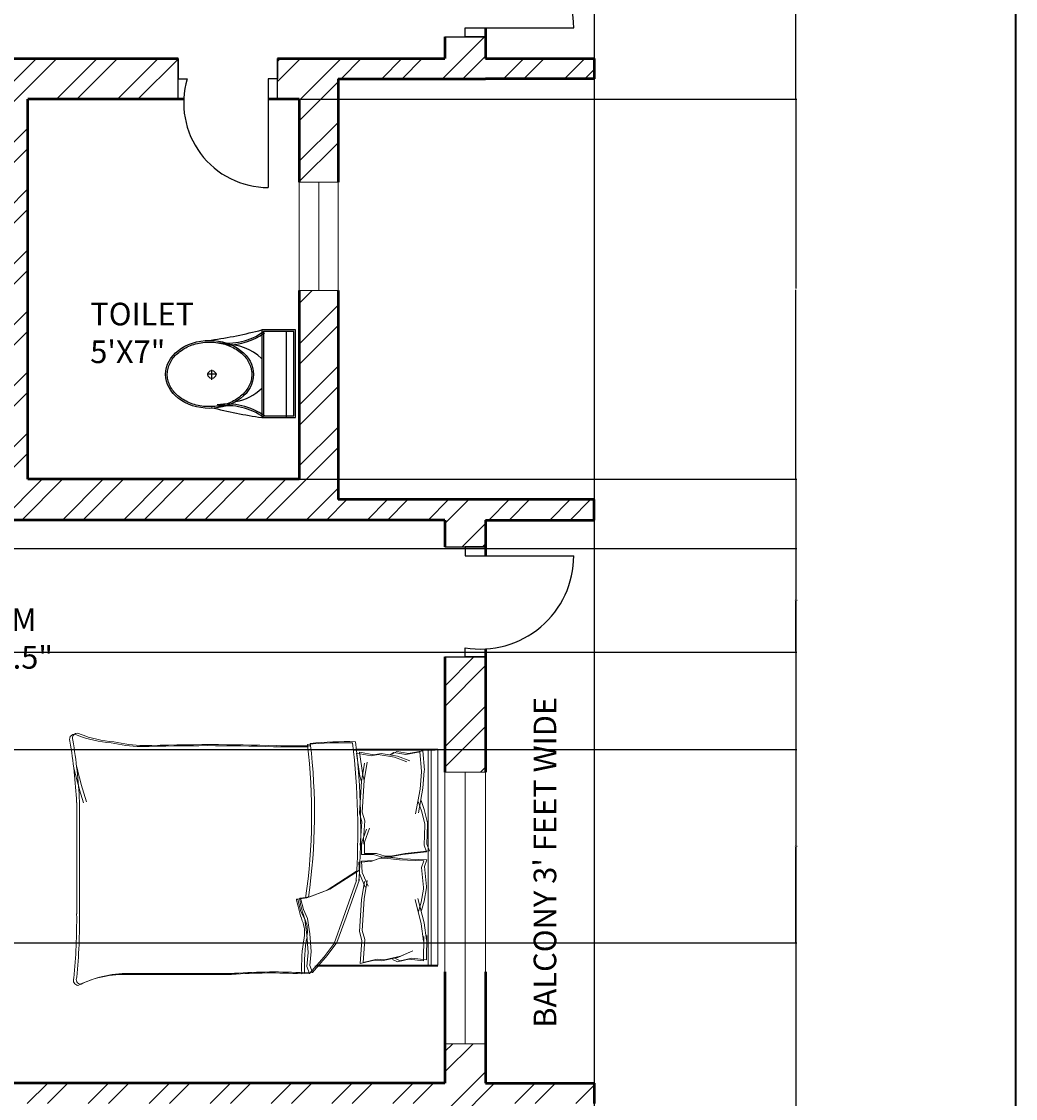
# Model space of a CAD drawing. Units: inches. Extents: x 1980 to 2738, y 1471 to 2568.
# Tile 15 of 22: x 2519 to 2738, y 1874 to 2112. Entities that reach past the tile are written whole.
import ezdxf

# ---------------------------------------------------------------- set-up
doc = ezdxf.new("R2010")
doc.units = ezdxf.units.IN
for name, color, linetype, lineweight in [('A-ANNO-DIMS', 2, 'Continuous', 18), ('A-ANNO-TTLB', 7, 'Continuous', 35), ('A-AREA-IDEN', 7, 'Continuous', 18), ('A-DOOR', 31, 'Continuous', 25), ('A-FLOR-BALC', 7, 'Continuous', 25), ('A-FLOR-FIXT', 8, 'Continuous', 25), ('A-FURN', 8, 'Continuous', 18), ('A-GLAZ', 141, 'Continuous', 18), ('A-WALL', 7, 'Continuous', 50)]:
    doc.layers.add(name, color=color, linetype=linetype, lineweight=lineweight)
doc.layers.add('A-WALL-PATT', color=9, linetype='Continuous', lineweight=13, true_color=0xd19cc7)
doc.styles.get("Standard").update_dxf_attribs({"font": 'arial.ttf'})
doc.dimstyles.get("Standard").update_dxf_attribs({"dimtxt": 0.18, "dimasz": 0.18, "dimexe": 0.18, "dimexo": 0.0625, "dimgap": 0.09, "dimtad": 0, "dimtih": 1, "dimtoh": 1, "dimdec": 4, "dimzin": 0, "dimdsep": 46, "dimtxsty": 'Standard', "dimcen": 0.09, "dimadec": 0, "dimazin": 0, "dimtfac": 1, "dimtdec": 4, "dimtofl": 0, "dimtmove": 0, "dimatfit": 3, "dimfxl": 1, "dimtolj": 1, "dimtzin": 0, "dimarcsym": 0})

# ---------------------------------------------------------------- blocks, each defined once
blk = doc.blocks.new('A$C31115884')
for p, q in [((257.5, 466.4), (257.5, 523.2)), ((283.1, 497.7), (223.4, 497.7)), ((0, 200), (0, 0)), ((520, 200), (0, 200)), ((520, 0), (520, 200)), ((10, 190), (10, 10)), ((510, 190), (10, 190)), ((510, 10), (510, 190)), ((510, 54.5), (0, 54.5)), ((10, 10), (510, 10)), ((0, 0), (520, 0))]:
    blk.add_line(p, q)
blk.add_circle((255.6, 496.4), 23.6)
for centre, radius, start, end in [((2777.7, -204.6), 2807, 165.4549, 171.71327), ((-294.5, 403.3), 364.7, 324.20913, 9.34987), ((-294.5, 403.3), 374.7, 324.20913, 9.34987), ((805.8, 403.3), 364.7, 170.65013, 215.79087), ((3237, 905), 2807, 188.28673, 194.5451), ((139.5, 406.2), 293.5, 315.84364, 2.65635), ((805.8, 403.3), 374.7, 179.20365, 215.79087), ((383.6, 406.2), 293.5, 190.27735, 224.15636)]:
    blk.add_arc(centre, radius, start, end)
blk.add_ellipse((256.2, 509.9), major_axis=(0, -260.7), ratio=0.772727)
blk.add_open_spline([(256.2, 259.2), (263.1, 259.2), (270, 259.7), (287.8, 262.3), (298.7, 265.1), (319.9, 273.1), (330.2, 278.4), (350.1, 291.1), (359.7, 298.7), (377.7, 315.9), (386.2, 325.5), (401.7, 346.6), (408.8, 358.1), (421.3, 382.5), (426.8, 395.5), (435.9, 422.4), (439.5, 436.4), (444.8, 465.1), (446.5, 479.7), (447.9, 509.2), (447.6, 524), (445, 553.3), (442.7, 567.8), (436.3, 596), (432.1, 609.7), (421.9, 636), (416, 648.6), (402.5, 672.1), (395, 683), (378.6, 703), (369.8, 712.1), (351.1, 728), (341.3, 734.8), (320.9, 746.2), (310.4, 750.7), (288.9, 757.3), (278, 759.4), (256, 761), (245, 760.6), (223.1, 757.2), (212.3, 754.3), (191.1, 746.1), (180.8, 740.7), (160.9, 727.8), (151.4, 720.1), (133.5, 702.7), (125.1, 693), (109.6, 671.7), (102.6, 660.2), (90.2, 635.7), (84.9, 622.7), (76, 595.6), (72.4, 581.6), (67.2, 552.9), (65.6, 538.2), (64.4, 508.8), (64.8, 494), (67.5, 464.7), (69.9, 450.2), (76.6, 422), (80.8, 408.3), (91.1, 382.2), (97.2, 369.7), (110.8, 346.3), (118.4, 335.4), (134.8, 315.6), (143.7, 306.7), (162.4, 290.9), (172.3, 284.2), (192.8, 273), (203.3, 268.6), (224.8, 262.2), (235.8, 260.2), (249.9, 259.3), (253, 259.2), (256.2, 259.2)], degree=3, knots=[0, 0, 0, 0, 0.110105, 0.110105, 0.285049, 0.285049, 0.459994, 0.459994, 0.634938, 0.634938, 0.809882, 0.809882, 0.984827, 0.984827, 1.159771, 1.159771, 1.334715, 1.334715, 1.50966, 1.50966, 1.684604, 1.684604, 1.859549, 1.859549, 2.034493, 2.034493, 2.209437, 2.209437, 2.384382, 2.384382, 2.559326, 2.559326, 2.73427, 2.73427, 2.909215, 2.909215, 3.084159, 3.084159, 3.259103, 3.259103, 3.434048, 3.434048, 3.608992, 3.608992, 3.783936, 3.783936, 3.958881, 3.958881, 4.133825, 4.133825, 4.30877, 4.30877, 4.483714, 4.483714, 4.658658, 4.658658, 4.833603, 4.833603, 5.008547, 5.008547, 5.183491, 5.183491, 5.358436, 5.358436, 5.53338, 5.53338, 5.708324, 5.708324, 5.883269, 5.883269, 6.058213, 6.058213, 6.233158, 6.233158, 6.283185, 6.283185, 6.283185, 6.283185])
blk = doc.blocks.new('BED-DOUBLE')
for p, q in [((27.75, 52.87), (24.5, 49.16)), ((27.75, 52.87), (24.5, 49.16)), ((28.38, 53.1), (25.13, 49.39)), ((28.38, 53.1), (25.13, 49.39)), ((29.49, 52.95), (27.75, 52.87, 3.87)), ((29.49, 52.95), (27.75, 52.87, 3.87)), ((28.36, 51.33), (27.75, 52.87)), ((28.36, 51.33), (27.75, 52.87)), ((30.13, 53.18), (28.38, 53.1, 3.87)), ((30.13, 53.18), (28.38, 53.1, 3.87)), ((29, 51.56), (28.38, 53.1)), ((29, 51.56), (28.38, 53.1)), ((0, 51.49), (0.64, 51.49)), ((0, 51.27), (26.61, 51.27)), ((0, 51.27), (26.61, 51.27)), ((0, 51.27), (0, 3.48)), ((0.64, 51.49), (27.25, 51.49)), ((0.64, 51.49), (27.25, 51.49)), ((1.53, 3.48), (1.53, 51.27)), ((1.53, 3.48), (1.53, 51.27)), ((2.17, 3.7), (2.17, 51.49)), ((2.17, 3.7), (2.17, 51.49)), ((2.56, 50.11), (2.46, 44.71)), ((2.56, 50.11), (2.46, 44.71)), ((2.56, 50.11), (5.77, 49.73)), ((2.56, 50.11), (5.77, 49.73)), ((3.2, 50.34), (3.1, 44.94)), ((3.2, 50.34), (3.1, 44.94)), ((3.2, 50.34), (6.41, 49.96)), ((3.2, 50.34), (6.41, 49.96)), ((5.77, 49.73), (8.34, 50.33)), ((5.77, 49.73), (8.34, 50.33)), ((6.41, 49.96), (8.98, 50.56)), ((6.41, 49.96), (8.98, 50.56)), ((11.83, 50.11), (8.26, 49.31)), ((11.83, 50.11), (8.26, 49.31)), ((8.34, 50.33), (9.38, 49.81)), ((8.34, 50.33), (9.38, 49.81)), ((12.47, 50.34), (8.9, 49.54)), ((12.47, 50.34), (8.9, 49.54)), ((8.98, 50.56), (10.02, 50.04)), ((8.98, 50.56), (10.02, 50.04)), ((13.43, 49.92), (11.83, 50.11)), ((13.43, 49.92), (11.83, 50.11)), ((14.07, 50.15), (12.47, 50.34)), ((14.07, 50.15), (12.47, 50.34)), ((16.57, 50.7), (13.43, 49.92)), ((16.57, 50.7), (13.43, 49.92)), ((17.21, 50.93), (14.07, 50.15)), ((17.21, 50.93), (14.07, 50.15)), ((16.17, 45.57), (16.57, 50.7)), ((16.17, 45.57), (16.57, 50.7)), ((16.81, 45.8), (17.21, 50.93)), ((16.81, 45.79), (17.21, 50.93)), ((28.06, 48.23), (28.36, 51.33)), ((28.06, 48.23), (28.36, 51.33)), ((28.69, 48.46), (29, 51.56)), ((28.69, 48.46), (29, 51.56)), ((8.26, 49.31), (5.58, 48.13)), ((8.26, 49.31), (5.58, 48.13)), ((8.9, 49.54), (6.22, 48.36)), ((8.9, 49.54), (6.22, 48.36)), ((24.5, 49.16), (22.33, 46.22)), ((24.5, 49.16), (22.33, 46.22)), ((25.13, 49.39), (22.97, 46.45)), ((25.13, 49.39), (22.97, 46.45)), ((28.36, 44.36), (28.06, 48.23)), ((28.36, 44.36), (28.06, 48.23)), ((29, 44.59), (28.69, 48.46)), ((29, 44.59), (28.69, 48.46)), ((2.46, 44.71), (2.54, 45.71)), ((2.46, 44.71), (2.54, 45.71)), ((2.54, 45.71), (3.07, 41.91)), ((2.54, 45.71), (3.07, 41.91)), ((3.1, 44.94), (3.18, 45.94)), ((3.1, 44.94), (3.18, 45.94)), ((3.18, 45.94), (3.71, 42.14)), ((3.18, 45.94), (3.71, 42.14)), ((16.73, 43.61), (16.17, 45.57)), ((16.73, 43.61), (16.17, 45.57)), ((17.37, 43.83), (16.81, 45.8)), ((17.37, 43.83), (16.81, 45.79)), ((22.33, 46.22), (20.32, 40.64)), ((22.33, 46.22), (20.32, 40.64)), ((22.97, 46.45), (20.96, 40.87)), ((22.97, 46.45), (20.96, 40.87)), ((16.29, 36.6), (16.73, 43.61)), ((16.29, 36.6), (16.73, 43.61)), ((16.93, 36.82), (17.37, 43.83)), ((16.93, 36.82), (17.37, 43.83)), ((28.83, 40.95), (28.36, 44.36)), ((28.83, 40.95), (28.36, 44.36)), ((29.47, 41.18), (29, 44.59)), ((29.47, 41.18), (29, 44.59)), ((3.07, 41.91), (4.42, 36.5)), ((3.07, 41.91), (4.42, 36.5)), ((3.71, 42.14), (5.06, 36.72)), ((3.71, 42.14), (5.06, 36.72)), ((20.32, 40.64), (17.38, 32.31)), ((20.32, 40.64), (17.38, 32.31)), ((20.96, 40.87), (18.02, 32.53)), ((20.96, 40.87), (18.02, 32.53)), ((29.76, 38.94), (28.83, 40.95)), ((29.76, 38.94), (28.83, 40.95)), ((30.4, 39.17), (29.47, 41.18)), ((30.4, 39.17), (29.47, 41.18)), ((3.67, 39.2), (3.08, 37.14)), ((3.67, 39.2), (3.08, 37.14)), ((4.31, 39.43), (3.72, 37.36)), ((4.31, 39.43), (3.72, 37.36)), ((30.38, 36.46), (29.76, 38.94)), ((30.38, 36.46), (29.76, 38.94)), ((31.02, 36.69), (30.4, 39.17)), ((31.02, 36.69), (30.4, 39.17)), ((79.24, 15.06), (79.24, 39.68)), ((79.24, 15.06), (79.24, 39.68)), ((79.88, 15.29), (79.88, 39.91)), ((79.88, 15.29), (79.88, 39.91)), ((3.08, 37.14), (2.54, 34.2)), ((3.08, 37.14), (2.54, 34.2)), ((3.72, 37.36), (3.18, 34.43)), ((3.72, 37.36), (3.18, 34.43)), ((15.63, 32.56), (16.29, 36.6)), ((15.63, 32.56), (16.29, 36.6)), ((16.27, 32.79), (16.93, 36.82)), ((16.27, 32.79), (16.93, 36.82)), ((23.88, 34.45), (28.36, 36.15)), ((23.88, 34.45), (28.36, 36.15)), ((24.52, 34.68), (29, 36.38)), ((24.52, 34.68), (29, 36.38)), ((28.36, 36.15), (30.38, 36.46)), ((28.36, 36.15), (30.38, 36.46)), ((29, 36.38), (31.02, 36.69)), ((29, 36.38), (31.02, 36.69)), ((2.54, 34.2), (2.56, 33.88)), ((2.54, 34.2), (2.56, 33.88)), ((2.56, 33.88), (2.98, 29.46)), ((2.56, 33.88), (2.98, 29.46)), ((3.18, 34.43), (3.2, 34.11)), ((3.18, 34.43), (3.2, 34.11)), ((3.2, 34.11), (3.62, 29.68)), ((3.2, 34.11), (3.62, 29.68)), ((16.74, 30.75), (15.45, 33.82)), ((16.74, 30.75), (15.45, 33.82)), ((17.38, 30.98), (16.09, 34.05)), ((17.38, 30.98), (16.09, 34.05)), ((17.38, 30.26), (23.88, 34.45)), ((17.38, 30.26), (23.88, 34.45)), ((18.02, 30.49), (24.52, 34.68)), ((18.02, 30.49), (24.52, 34.68)), ((17.53, 28.53), (17.38, 30.98)), ((17.53, 28.53), (17.38, 30.98)), ((2.98, 29.46), (2.49, 27.98)), ((2.98, 29.46), (2.49, 27.98)), ((3.62, 29.68), (3.13, 28.21)), ((3.62, 29.68), (3.13, 28.21)), ((16.89, 28.3), (16.74, 30.75)), ((16.89, 28.3), (16.74, 30.75)), ((1.87, 25.98), (7.22, 26.56)), ((1.87, 25.98), (7.22, 26.56)), ((2.49, 27.98), (7.87, 27.73)), ((2.49, 27.98), (7.87, 27.73)), ((2.51, 26.21), (7.86, 26.79)), ((2.51, 26.21), (7.86, 26.79)), ((3.09, 24.77), (2.51, 26.21)), ((3.09, 24.77), (2.51, 26.21)), ((3.13, 28.21), (8.51, 27.96)), ((3.13, 28.21), (8.51, 27.96)), ((7.22, 26.56), (10.4, 27.14)), ((7.22, 26.56), (10.4, 27.14)), ((7.86, 26.79), (11.04, 27.37)), ((7.86, 26.79), (11.04, 27.37)), ((7.87, 27.73), (11.08, 27.36)), ((7.87, 27.73), (11.08, 27.35)), ((8.51, 27.96), (11.72, 27.58)), ((8.51, 27.96), (11.72, 27.58)), ((10.4, 27.14), (11.7, 27.14)), ((10.4, 27.14), (11.7, 27.14)), ((11.04, 27.37), (12.34, 27.37)), ((11.04, 27.37), (12.34, 27.37)), ((11.08, 27.36), (12.38, 27.44)), ((11.08, 27.35), (12.38, 27.44)), ((11.7, 27.14), (13.58, 26.56)), ((11.7, 27.14), (13.58, 26.56)), ((11.72, 27.58), (13.02, 27.66)), ((11.72, 27.58), (13.02, 27.66)), ((12.34, 27.37), (14.22, 26.79)), ((12.34, 27.37), (14.22, 26.79)), ((12.38, 27.44), (14.22, 28.13)), ((12.38, 27.44), (14.22, 28.13)), ((13.02, 27.66), (14.86, 28.36)), ((13.02, 27.66), (14.86, 28.36)), ((13.58, 26.56), (16.26, 26.56)), ((13.58, 26.56), (16.26, 26.56)), ((14.22, 28.13), (16.89, 28.3)), ((14.22, 28.13), (16.89, 28.3)), ((14.22, 26.79), (16.9, 26.79)), ((14.22, 26.79), (16.9, 26.79)), ((14.86, 28.36), (17.53, 28.53)), ((14.86, 28.36), (17.53, 28.53)), ((16.26, 26.56), (16.26, 24.1)), ((16.26, 26.56), (16.26, 24.1)), ((16.9, 26.79), (16.9, 24.33)), ((16.9, 26.79), (16.9, 24.33)), ((2.45, 24.54), (1.87, 25.98)), ((2.45, 24.54), (1.87, 25.98)), ((2.3, 20.09), (2.45, 24.54)), ((2.3, 20.09), (2.45, 24.54)), ((2.94, 20.32), (3.09, 24.77)), ((2.94, 20.32), (3.09, 24.77)), ((16.26, 24.1), (15.17, 20.96)), ((16.26, 24.1), (15.17, 20.96)), ((16.9, 24.33), (15.81, 21.19)), ((16.9, 24.33), (15.81, 21.19)), ((16.17, 19.38), (16.57, 24.52)), ((16.17, 19.38), (16.57, 24.52)), ((16.81, 19.61), (17.21, 24.74)), ((16.81, 19.61), (17.21, 24.74)), ((2.3, 19.77), (2.3, 20.09)), ((2.3, 19.77), (2.3, 20.09)), ((3.03, 16.88), (2.3, 19.77)), ((3.03, 16.88), (2.3, 19.77)), ((2.94, 20), (2.94, 20.32)), ((2.94, 20), (2.94, 20.32)), ((3.67, 17.11), (2.94, 20)), ((3.67, 17.11), (2.94, 20)), ((16.73, 17.42), (16.17, 19.38)), ((16.73, 17.42), (16.17, 19.38)), ((17.37, 17.65), (16.81, 19.61)), ((17.37, 17.65), (16.81, 19.61)), ((3.75, 14.86), (3.03, 16.88)), ((3.75, 14.85), (3.03, 16.88)), ((3.32, 12.11), (4.33, 17.6)), ((3.32, 12.11), (4.33, 17.6)), ((4.39, 15.08), (3.67, 17.11)), ((4.39, 15.08), (3.67, 17.11)), ((3.96, 12.34), (4.97, 17.83)), ((3.96, 12.34), (4.97, 17.83)), ((16.29, 10.41), (16.73, 17.42)), ((16.29, 10.41), (16.73, 17.42)), ((16.93, 10.64), (17.37, 17.65)), ((16.93, 10.64), (17.37, 17.65)), ((3.03, 8.29), (3.32, 12.11)), ((3.03, 8.28), (3.32, 12.11)), ((3.67, 8.51), (3.96, 12.34)), ((3.67, 8.51), (3.96, 12.34)), ((15.63, 6.38), (16.29, 10.41)), ((15.63, 6.38), (16.29, 10.41)), ((16.27, 6.61), (16.93, 10.64)), ((16.27, 6.61), (16.93, 10.64)), ((16.29, 10.41), (16.62, 9.28)), ((16.29, 10.41), (16.62, 9.28)), ((16.93, 10.64), (17.26, 9.51)), ((16.93, 10.64), (17.26, 9.51)), ((3.01, 8.18), (3.03, 8.29)), ((3.01, 8.18), (3.03, 8.28)), ((3.34, 3.9), (3.01, 8.18)), ((3.34, 3.9), (3.01, 8.18)), ((3.65, 8.41), (3.67, 8.51)), ((3.65, 8.41), (3.67, 8.51)), ((3.98, 4.13), (3.65, 8.41)), ((3.98, 4.13), (3.65, 8.41)), ((16.62, 9.28), (17.34, 4.18)), ((16.62, 9.28), (17.34, 4.18)), ((17.26, 9.51), (17.98, 4.41)), ((17.26, 9.51), (17.98, 4.41)), ((8.95, 5.05), (6.21, 6.06)), ((8.95, 5.05), (6.21, 6.06)), ((9.59, 5.28), (6.85, 6.29)), ((9.59, 5.28), (6.85, 6.29)), ((12.57, 4.47), (8.95, 5.05)), ((12.57, 4.47), (8.95, 5.05)), ((13.21, 4.7), (9.59, 5.28)), ((13.21, 4.7), (9.59, 5.28)), ((9.74, 4.27), (10.75, 4.85)), ((9.74, 4.27), (10.75, 4.85)), ((14.16, 4.76), (12.57, 4.47)), ((14.16, 4.76), (12.57, 4.47)), ((14.8, 4.99), (13.21, 4.7)), ((14.8, 4.99), (13.21, 4.7)), ((17.34, 4.18), (14.16, 4.76)), ((17.34, 4.18), (14.16, 4.76)), ((17.98, 4.41), (14.8, 4.99)), ((17.98, 4.41), (14.8, 4.99)), ((18.11, 3.48), (0, 3.48)), ((18.11, 3.48), (0, 3.48)), ((18.75, 3.7), (0.64, 3.7)), ((18.75, 3.7), (0.64, 3.7)), ((3.32, 3.89), (6.5, 4.47)), ((3.32, 3.89), (6.5, 4.47)), ((3.96, 4.12), (7.14, 4.7)), ((3.96, 4.12), (7.14, 4.7)), ((6.5, 4.47), (9.1, 4.04)), ((6.5, 4.47), (9.1, 4.04)), ((7.14, 4.7), (9.74, 4.27)), ((7.14, 4.7), (9.74, 4.27)), ((9.1, 4.04), (10.11, 4.62)), ((9.1, 4.04), (10.11, 4.62))]:
    blk.add_line(p, q)
for centre, radius, start, end in [((68.67, 76.16), 23.07, 267.4714, 296.4681), ((68.67, 76.16), 23.07, 267.4714, 296.4681), ((69.31, 76.39), 23.07, 267.4714, 296.4681), ((69.31, 76.39), 23.07, 267.4714, 296.4681), ((78.87, 54.41), 1.1, 332.6588, 86.02), ((78.87, 54.41), 1.1, 332.6588, 86.02), ((79.51, 54.64), 1.1, 332.6588, 86.02), ((79.51, 54.64), 1.1, 332.6588, 86.02), ((-6.66, 51.33), 36.18, 349.8763, 2.5657), ((-6.66, 51.33), 36.18, 349.8763, 2.5657), ((36.31, 182.27), 129.5, 266.9791, 273.8365), ((36.31, 182.27), 129.5, 266.9791, 273.8365), ((-6.02, 51.56), 36.18, 349.8763, 2.5657), ((-6.02, 51.56), 36.18, 349.8763, 2.5657), ((36.95, 182.49), 129.5, 266.9791, 273.8365), ((36.95, 182.49), 129.5, 266.9791, 273.8365), ((67.82, -4508.74), 4561.86, 90.00217, 90.28689), ((67.82, -4508.74), 4561.86, 90.00217, 90.28689), ((68.46, -4508.51), 4561.86, 90.00217, 90.28689), ((68.46, -4508.52), 4561.86, 90.00217, 90.28689), ((212.28, 41.15), 133.04, 174.4998, 180.6351), ((212.28, 41.15), 133.04, 174.4998, 180.6351), ((212.92, 41.38), 133.04, 174.4998, 180.6351), ((212.92, 41.38), 133.04, 174.4998, 180.6351), ((35.07, 43.74), 6.22, 168.6608, 203.7384), ((35.07, 43.74), 6.22, 168.6608, 203.7384), ((35.71, 43.97), 6.22, 168.6608, 203.7384), ((35.71, 43.97), 6.22, 168.6608, 203.7384), ((1.48, 31.15), 29.65, 10.6617, 19.8806), ((1.48, 31.15), 29.65, 10.6617, 19.8806), ((2.12, 31.38), 29.65, 10.6617, 19.8806), ((2.12, 31.38), 29.65, 10.6617, 19.8806), ((156.32, 17.76), 129.02, 171.7845, 186.9006), ((156.32, 17.76), 129.02, 171.7845, 186.9006), ((156.96, 17.98), 129.02, 171.7845, 186.9006), ((156.96, 17.98), 129.02, 171.7845, 186.9006), ((30.44, 36.64), 0.185, 250.2464, 1.1377), ((30.44, 36.64), 0.185, 250.2464, 1.1377), ((31.08, 36.86), 0.185, 250.2464, 1.1377), ((31.08, 36.86), 0.185, 250.2464, 1.1377), ((182.05, 21.36), 164.97, 176.0865, 186.7821), ((182.05, 21.36), 164.97, 176.0865, 186.7821), ((182.69, 21.59), 164.97, 176.0865, 186.7821), ((182.69, 21.59), 164.97, 176.0865, 186.7821), ((-23.71, -17.22), 106.46, 13.3832, 17.7053), ((-23.71, -17.22), 106.46, 13.3832, 17.7053), ((-23.07, -16.99), 106.46, 13.3832, 17.7053), ((-23.07, -16.99), 106.46, 13.3832, 17.7053), ((200.84, 21.43), 121.76, 182.9958, 189.4091), ((200.84, 21.43), 121.76, 182.9958, 189.4091), ((201.48, 21.66), 121.76, 182.9958, 189.4091), ((201.48, 21.66), 121.76, 182.9958, 189.4091), ((20.74, 85.39), 83.31, 268.7218, 275.604), ((20.74, 85.39), 83.31, 268.7218, 275.604), ((31.17, -167.31), 170.11, 88.4762, 91.0082), ((31.17, -167.31), 170.11, 88.4762, 91.0082), ((31.81, -167.08), 170.11, 88.4762, 91.0082), ((31.81, -167.08), 170.11, 88.4762, 91.0082), ((50.61, 484.82), 482.31, 268.2277, 271.7185), ((50.61, 484.82), 482.31, 268.2277, 271.7185), ((51.25, 485.05), 482.31, 268.2277, 271.7185), ((51.25, 485.05), 482.31, 268.2277, 271.7185), ((64.51, -26.9), 29.63, 76.0648, 88.9113), ((64.51, -26.9), 29.63, 76.0648, 88.9113), ((65.15, -26.67), 29.63, 76.0648, 88.9113), ((65.15, -26.67), 29.63, 76.0648, 88.9113), ((20.1, 85.16), 83.31, 268.7218, 275.604), ((20.1, 85.16), 83.31, 268.7218, 275.604), ((70.28, -21.66), 23.56, 67.9751, 86.652), ((70.28, -21.66), 23.56, 67.9751, 86.652), ((70.91, -21.43), 23.56, 67.9751, 86.652), ((70.91, -21.43), 23.56, 67.9751, 86.652), ((79.72, 1.09), 1.09, 236.1736, 23.4781), ((79.72, 1.09), 1.09, 236.1736, 23.4781), ((80.36, 1.32), 1.09, 236.1736, 23.4781), ((80.36, 1.32), 1.09, 236.1736, 23.4781)]:
    blk.add_arc(centre, radius, start, end)
blk = doc.blocks.new('*D37')
at = {"layer": 'A-ANNO-DIMS', "color": 0, "lineweight": -2, "transparency": 16777216}
for p, q in [((2579.97, 2011.21), (2689.91, 2011.21)), ((2689.73, 2011.03), (2689.73, 1827.64)), ((2689.73, 1643.89), (2689.73, 1827.27)), ((2621.15, 1643.71), (2689.91, 1643.71))]:
    blk.add_line(p, q, dxfattribs=at)
at = {"layer": 'A-ANNO-DIMS', "color": 0, "transparency": 16777216}
for points in [[(2689.7, 2011.03), (2689.76, 2011.03), (2689.73, 2011.21)], [(2689.7, 1643.89), (2689.76, 1643.89), (2689.73, 1643.71)]]:
    blk.add_solid(points, dxfattribs=at)
at = {"layer": 'Defpoints', "color": 0, "transparency": 16777216}
for p in [(2579.9, 2011.21), (2689.73, 2011.21), (2621.08, 1643.71)]:
    blk.add_point(p, dxfattribs=at)
at = {"layer": 'A-ANNO-DIMS', "color": 0, "transparency": 16777216, "insert": (2689.73, 1827.46), "char_height": 0.18, "attachment_point": 5}
blk.add_mtext('\\A1;367.5', dxfattribs=at)
blk = doc.blocks.new('*D38')
at = {"layer": 'A-ANNO-DIMS', "color": 0, "lineweight": -2, "transparency": 16777216}
for p, q in [((2579.97, 2095.21), (2689.91, 2095.21)), ((2689.73, 2095.03), (2689.73, 2053.39)), ((2689.73, 2011.39), (2689.73, 2053.02)), ((2579.97, 2011.21), (2689.91, 2011.21))]:
    blk.add_line(p, q, dxfattribs=at)
at = {"layer": 'A-ANNO-DIMS', "color": 0, "transparency": 16777216}
for points in [[(2689.7, 2095.03), (2689.76, 2095.03), (2689.73, 2095.21)], [(2689.7, 2011.39), (2689.76, 2011.39), (2689.73, 2011.21)]]:
    blk.add_solid(points, dxfattribs=at)
at = {"layer": 'Defpoints', "color": 0, "transparency": 16777216}
for p in [(2579.9, 2095.21), (2689.73, 2095.21), (2579.9, 2011.21)]:
    blk.add_point(p, dxfattribs=at)
at = {"layer": 'A-ANNO-DIMS', "color": 0, "transparency": 16777216, "insert": (2689.73, 2053.21), "char_height": 0.18, "attachment_point": 5}
blk.add_mtext('\\A1;84', dxfattribs=at)
blk = doc.blocks.new('*D39')
at = {"layer": 'A-ANNO-DIMS', "color": 0, "lineweight": -2, "transparency": 16777216}
for p, q in [((2621.15, 2462.71), (2689.91, 2462.71)), ((2689.73, 2462.53), (2689.73, 2279.14)), ((2689.73, 2095.39), (2689.73, 2278.77)), ((2579.97, 2095.21), (2689.91, 2095.21))]:
    blk.add_line(p, q, dxfattribs=at)
at = {"layer": 'A-ANNO-DIMS', "color": 0, "transparency": 16777216}
for points in [[(2689.7, 2462.53), (2689.76, 2462.53), (2689.73, 2462.71)], [(2689.7, 2095.39), (2689.76, 2095.39), (2689.73, 2095.21)]]:
    blk.add_solid(points, dxfattribs=at)
at = {"layer": 'Defpoints', "color": 0, "transparency": 16777216}
for p in [(2621.08, 2462.71), (2689.73, 2462.71), (2579.9, 2095.21)]:
    blk.add_point(p, dxfattribs=at)
at = {"layer": 'A-ANNO-DIMS', "color": 0, "transparency": 16777216, "insert": (2689.73, 2278.96), "char_height": 0.18, "attachment_point": 5}
blk.add_mtext('\\A1;367.5', dxfattribs=at)
blk = doc.blocks.new('*D55')
at = {"layer": 'A-ANNO-DIMS', "color": 0, "lineweight": -2, "transparency": 16777216}
for p, q in [((2269.76, 1951.46), (2689.91, 1951.46)), ((2689.73, 1951.28), (2689.73, 1930.28)), ((2689.73, 1908.91), (2689.73, 1929.91)), ((2269.76, 1908.73), (2689.91, 1908.73))]:
    blk.add_line(p, q, dxfattribs=at)
at = {"layer": 'A-ANNO-DIMS', "color": 0, "transparency": 16777216}
for points in [[(2689.7, 1951.28), (2689.76, 1951.28), (2689.73, 1951.46)], [(2689.7, 1908.91), (2689.76, 1908.91), (2689.73, 1908.73)]]:
    blk.add_solid(points, dxfattribs=at)
at = {"layer": 'Defpoints', "color": 0, "transparency": 16777216}
for p in [(2269.7, 1951.46), (2689.73, 1951.46), (2269.7, 1908.73)]:
    blk.add_point(p, dxfattribs=at)
at = {"layer": 'A-ANNO-DIMS', "color": 0, "transparency": 16777216, "insert": (2689.73, 1930.09), "char_height": 0.18, "attachment_point": 5}
blk.add_mtext('\\A1;42.735', dxfattribs=at)
blk = doc.blocks.new('*D56')
at = {"layer": 'A-ANNO-DIMS', "color": 0, "lineweight": -2, "transparency": 16777216}
for p, q in [((2114.15, 1995.93), (2689.91, 1995.93)), ((2689.73, 1995.75), (2689.73, 1984.65)), ((2689.73, 1973.18), (2689.73, 1984.28)), ((2114.15, 1973), (2689.91, 1973))]:
    blk.add_line(p, q, dxfattribs=at)
at = {"layer": 'A-ANNO-DIMS', "color": 0, "transparency": 16777216}
for points in [[(2689.7, 1995.75), (2689.76, 1995.75), (2689.73, 1995.93)], [(2689.7, 1973.18), (2689.76, 1973.18), (2689.73, 1973)]]:
    blk.add_solid(points, dxfattribs=at)
at = {"layer": 'Defpoints', "color": 0, "transparency": 16777216}
for p in [(2114.08, 1995.93), (2689.73, 1995.93), (2114.08, 1973)]:
    blk.add_point(p, dxfattribs=at)
at = {"layer": 'A-ANNO-DIMS', "color": 0, "transparency": 16777216, "insert": (2689.73, 1984.47), "char_height": 0.18, "attachment_point": 5}
blk.add_mtext('\\A1;22.935', dxfattribs=at)

msp = doc.modelspace()

# ---------------------------------------------------------------- hatches: boundary and pattern name
at = {"layer": 'A-WALL-PATT'}
h = msp.add_hatch(dxfattribs=at)
h.set_pattern_fill('ANSI32', color=256)
h.paths.add_polyline_path([(2257.5661, 2416.2064), (2257.5661, 2420.7064), (2250.5833, 2420.7064), (2250.5833, 2462.7064), (2246.0833, 2462.7064), (2246.0833, 2420.7064), (2237.0791, 2420.7064), (2237.0791, 2411.7064), (2246.0833, 2411.7064), (2246.0833, 2291.7064), (2242.6109, 2291.7064), (2242.6109, 2287.2064), (2246.0833, 2287.2064), (2250.5833, 2287.2064), (2250.5833, 2291.7064), (2250.5833, 2411.7064), (2257.5661, 2411.7064)])
h.paths.add_polyline_path([(2387.0396, 2416.2064), (2387.0396, 2420.7064), (2367.5833, 2420.7064), (2367.5833, 2462.7064), (2358.5833, 2462.7064), (2358.5833, 2420.7064), (2329.3087, 2420.7064), (2329.3087, 2411.7064), (2358.5833, 2411.7064), (2358.5833, 2321.7275), (2358.5833, 2309.7064), (2347.3089, 2309.7064), (2293.3089, 2309.7064), (2293.3089, 2259.0771), (2297.8089, 2259.0771), (2297.8089, 2305.2064), (2347.3089, 2305.2064), (2347.3089, 2284.7412), (2351.8089, 2284.7412), (2351.8089, 2305.2064), (2372.3188, 2305.2064), (2372.3761, 2284.3899), (2377.0295, 2284.3899), (2377.0295, 2299.3058), (2377.0295, 2305.2064), (2426.5295, 2305.2064), (2426.5295, 2257.5573), (2431.0295, 2257.5573), (2431.0295, 2309.7064), (2377.0295, 2309.7064), (2367.5833, 2309.7064), (2367.5833, 2321.7275), (2367.5833, 2411.7064), (2387.0396, 2411.7064)])
h.paths.add_polyline_path([(2448.5267, 2416.2064), (2448.5267, 2420.7064), (2423.0396, 2420.7064), (2423.0396, 2411.7064), (2448.5267, 2411.7064)])
h.paths.add_polyline_path([(2130.9128, 2416.2064), (2130.9128, 2420.7064), (2105.0833, 2420.7064), (2105.0833, 2386.6942), (2114.0833, 2386.6942), (2114.0833, 2411.7064), (2130.9128, 2411.7064)])
h.paths.add_polyline_path([(2212.9478, 2420.7064), (2190.9128, 2420.7064), (2190.9128, 2411.7064), (2212.9478, 2411.7064), (2212.9478, 2416.2064)])
h.paths.add_polyline_path([(2114.0833, 2326.6942), (2105.0833, 2326.6942), (2105.0833, 2291.7064), (2081.0833, 2291.7064), (2081.0833, 2287.2064), (2105.0833, 2287.2064), (2105.0833, 2276.1935), (2114.0833, 2276.1935), (2114.0833, 2287.2064), (2166.3825, 2287.2064), (2166.3825, 2289.4564), (2166.3825, 2291.7064), (2114.0833, 2291.7064)])
h.paths.add_polyline_path([(2114.0833, 2252.1935), (2105.0833, 2252.1935), (2105.0833, 2233.2064), (2081.0833, 2233.2064), (2081.0833, 2228.7064), (2105.0833, 2228.7064), (2105.0833, 2213.4478), (2114.0833, 2213.4478), (2114.0833, 2228.7064), (2195.0833, 2228.7064), (2199.5833, 2228.7064), (2208.4455, 2228.7064), (2208.4455, 2230.9564), (2208.4455, 2233.2064), (2199.5833, 2233.2064), (2199.5833, 2287.2064), (2206.8904, 2287.2064), (2206.8904, 2289.4564), (2206.8904, 2291.7064), (2189.446, 2291.7064), (2189.446, 2289.4564), (2189.446, 2287.2064), (2195.0833, 2287.2064), (2195.0833, 2233.2064), (2114.0833, 2233.2064)])
h.paths.add_polyline_path([(2114.0833, 2153.4478), (2109.5833, 2153.4478), (2105.0833, 2153.4478), (2105.0833, 2135.2374), (2114.0833, 2135.2374)], flags=17)
h.paths.add_polyline_path([(2135.9619, 2095.4081), (2140.1805, 2095.4081), (2140.1805, 2104.2064), (2114.0833, 2104.2064), (2114.0833, 2110.3997), (2109.5833, 2110.3997), (2105.0833, 2110.3997), (2105.0833, 2104.2064), (2081.0833, 2104.2064), (2081.0833, 2099.7064), (2105.0833, 2099.7064), (2127.5416, 2099.8532), (2127.5416, 2056.9393), (2136.2133, 2056.9393)], flags=17)
h.paths.add_polyline_path([(2255.4895, 2104.2064), (2250.5833, 2104.2064), (2250.5833, 2233.2064), (2246.0833, 2233.2064), (2242.4941, 2233.2064), (2242.4941, 2228.7064), (2246.0833, 2228.7064), (2246.0833, 2104.2064), (2163.6825, 2104.2064), (2163.6825, 2099.8072), (2163.6825, 2095.4081), (2191.4325, 2095.4081), (2191.4325, 2011.2064), (2186.0833, 2011.2064), (2136.5143, 2010.8824), (2136.3702, 2032.9403), (2131.9559, 2032.9115), (2127.5416, 2032.8826), (2127.5416, 2006.7064), (2105.0833, 2006.7064), (2081.0833, 2006.7064), (2081.0833, 2002.2064), (2105.0833, 2002.2064), (2105.0833, 1995.9329), (2114.0833, 1995.9329), (2114.0833, 2002.2064), (2246.0833, 2002.2064), (2246.0833, 1877.7064), (2242.1358, 1877.7064), (2242.1358, 1873.2064), (2250.5833, 1873.2064), (2250.5833, 2002.2064), (2255.3335, 2002.2064), (2255.3335, 2011.2064), (2195.9325, 2011.2064), (2195.9325, 2095.2064), (2255.4895, 2095.2064), (2255.4895, 2099.5471)])
h.paths.add_polyline_path([(2199.5833, 1873.2064), (2209.827, 1873.2064), (2209.827, 1875.4564), (2209.827, 1877.7064), (2114.0833, 1877.7064), (2114.0833, 1890.0968), (2105.0833, 1890.0968), (2105.0833, 1877.7064), (2081.0833, 1877.7064), (2081.0833, 1873.2064), (2105.0833, 1873.2064), (2105.0833, 1857.7279), (2114.0833, 1857.7279), (2114.0833, 1873.2064), (2195.0833, 1873.2064), (2195.0833, 1819.2064), (2190.298, 1819.2064), (2190.298, 1814.7064), (2209.8976, 1814.7064), (2209.8976, 1816.9564), (2209.8976, 1819.2064), (2199.5833, 1819.2064)])
h.paths.add_polyline_path([(2114.0833, 1814.7064), (2166.2538, 1814.7064), (2166.2538, 1816.9564), (2166.2538, 1819.2064), (2114.0833, 1819.2064), (2114.0833, 1833.7279), (2109.5833, 1833.7279), (2105.0833, 1833.7279), (2105.0833, 1819.2064), (2081.0833, 1819.2064), (2081.0833, 1814.7064), (2105.0833, 1814.7064), (2105.0833, 1782.5516), (2114.0833, 1782.5516)])
h.paths.add_polyline_path([(2114.0833, 1722.5516), (2109.5833, 1722.5516), (2105.0833, 1722.5516), (2105.0833, 1685.7064), (2124.5104, 1685.7064), (2124.5104, 1690.2064), (2124.5104, 1694.7064), (2114.0833, 1694.7064)])
h.paths.add_polyline_path([(2218.8787, 1694.7064), (2184.5104, 1694.7064), (2184.5104, 1685.7064), (2218.8787, 1685.7064), (2218.8787, 1690.2064)])
h.paths.add_polyline_path([(2250.5833, 1819.2064), (2242.6431, 1819.2064), (2242.6431, 1816.9564), (2242.6431, 1814.7064), (2246.0833, 1814.7064), (2246.0833, 1694.7064), (2240.4035, 1694.7064), (2240.4035, 1690.2064), (2240.4035, 1685.7064), (2246.0833, 1685.7064), (2246.0833, 1643.7064), (2250.5833, 1643.7064), (2250.5833, 1685.7064), (2255.9859, 1685.7064), (2255.9859, 1690.2064), (2255.9859, 1694.7064), (2250.5833, 1694.7064)])
h.paths.add_polyline_path([(2297.4764, 1694.7064), (2279.3934, 1694.7064), (2279.3934, 1690.2064), (2279.3934, 1685.7064), (2297.4764, 1685.7064), (2297.4764, 1690.2064)])
h.paths.add_polyline_path([(2377.1596, 1694.7064), (2367.5833, 1694.7064), (2367.5833, 1787.7064), (2431.0295, 1787.7064), (2431.0295, 1792.2064), (2431.0295, 1849.4149), (2428.7795, 1849.4149), (2426.5295, 1849.4149), (2426.5295, 1792.2064), (2421.5833, 1792.2064), (2367.5833, 1792.2064), (2297.8089, 1792.2064), (2297.8089, 1850.2946), (2295.5589, 1850.2946), (2293.3089, 1850.2946), (2293.3089, 1792.2064), (2293.3089, 1787.7064), (2297.8089, 1787.7064), (2358.5833, 1787.7064), (2358.5833, 1694.7064), (2333.4764, 1694.7064), (2333.4764, 1685.7064), (2358.5833, 1685.7064), (2358.5833, 1643.7064), (2367.5833, 1643.7064), (2367.5833, 1685.7064), (2377.1596, 1685.7064)])
h.paths.add_polyline_path([(2442.4912, 1694.7064), (2413.1596, 1694.7064), (2413.1596, 1685.7064), (2442.4912, 1685.7064)])
h.paths.add_polyline_path([(2480.0833, 1814.7064), (2483.4816, 1814.7064), (2483.4816, 1817.9384), (2483.4816, 1819.2064), (2475.5833, 1819.2064), (2475.5833, 1694.7064), (2470.7283, 1694.7064), (2470.7283, 1685.7064), (2475.5833, 1685.7064), (2475.5833, 1643.7064), (2480.0833, 1643.7064), (2480.0833, 1685.7064), (2486.3293, 1685.7064), (2486.3293, 1690.2064), (2486.3293, 1694.7064), (2480.0833, 1694.7064)])
h.paths.add_polyline_path([(2621.0833, 1721.7349), (2612.0833, 1721.7349), (2612.0833, 1694.7064), (2586.1453, 1694.7064), (2586.1453, 1685.7064), (2621.0833, 1685.7064)])
h.paths.add_polyline_path([(2526.1453, 1690.2064), (2526.1453, 1694.7064), (2511.584, 1694.7064), (2511.584, 1690.2064), (2511.584, 1685.7064), (2526.1453, 1685.7064)])
h.paths.add_polyline_path([(2645.0833, 1819.2064), (2621.0833, 1819.2064), (2621.0833, 1835.8527), (2616.5833, 1835.8527), (2612.0833, 1835.8527), (2612.0833, 1819.2064), (2560.2541, 1819.2064), (2560.2541, 1814.7064), (2612.0833, 1814.7064), (2612.0833, 1781.7349), (2621.0833, 1781.7349), (2621.0833, 1814.7064), (2645.0833, 1814.7064)])
h.paths.add_polyline_path([(2645.0833, 1877.7064), (2621.0833, 1877.7064), (2621.0833, 1886.4375), (2612.0833, 1886.4375), (2612.0833, 1877.7064), (2517.1032, 1877.7064), (2517.1032, 1875.4564), (2517.1032, 1873.2064), (2526.5833, 1873.2064), (2526.5833, 1819.2064), (2516.6454, 1819.2064), (2516.6454, 1816.9564), (2516.6454, 1814.7064), (2536.4445, 1814.7064), (2536.4445, 1816.9564), (2536.4445, 1819.2064), (2531.0833, 1819.2064), (2531.0833, 1873.2064), (2612.0833, 1873.2064), (2612.0833, 1859.8527), (2621.0833, 1859.8527), (2621.0833, 1873.2064), (2645.0833, 1873.2064)])
h.paths.add_polyline_path([(2645.0833, 2006.7064), (2621.0833, 2006.7064), (2588.5085, 2006.7064), (2588.5085, 2052.9125), (2579.9045, 2052.9125), (2579.9045, 2011.2064), (2519.9045, 2011.2064), (2519.9045, 2095.2064), (2553.1204, 2095.2064), (2553.1204, 2104.2064), (2480.0833, 2104.2064), (2480.0833, 2228.7064), (2484.3832, 2228.7064), (2484.3832, 2230.9564), (2484.3832, 2233.2064), (2475.5833, 2233.2064), (2475.5833, 2104.2064), (2463.1308, 2104.2064), (2463.1308, 2095.2064), (2501.2463, 2095.2064), (2510.9045, 2095.2064), (2515.4045, 2095.2064), (2515.4045, 2011.2064), (2510.9045, 2011.2064), (2501.2463, 2011.2064), (2462.5957, 2011.2064), (2462.5957, 2002.2064), (2475.5833, 2002.2064), (2475.5833, 1873.2064), (2483.6146, 1873.2064), (2483.6146, 1875.4564), (2483.6146, 1877.7064), (2480.0833, 1877.7064), (2480.0833, 2002.2064), (2612.0833, 2002.2064), (2612.0833, 1996.309), (2621.0833, 1996.309), (2621.0833, 2002.2064), (2645.0833, 2002.2064)])
h.paths.add_polyline_path([(2588.5085, 2099.7277), (2621.0833, 2099.7277), (2645.0833, 2099.7064), (2645.0833, 2104.2064), (2621.0833, 2104.2064), (2621.0833, 2109.0038), (2616.5833, 2109.0038), (2612.0833, 2109.0038), (2612.0833, 2104.2064), (2575.0621, 2104.2064), (2575.0621, 2099.7064), (2575.0621, 2095.2064), (2579.9045, 2095.2064), (2579.9045, 2076.9125), (2588.5085, 2076.9125)], flags=17)
h.paths.add_polyline_path([(2367.5833, 2002.2064), (2373.7228, 2002.2064), (2373.7228, 2006.7064), (2373.7228, 2011.2064), (2350.7889, 2011.2064), (2350.7889, 2006.7064), (2350.7889, 2002.2064), (2358.5833, 2002.2064), (2358.5833, 1877.7064), (2293.3089, 1877.7064), (2293.3089, 1870.4987), (2297.8089, 1870.4987), (2297.8089, 1873.2064), (2347.3089, 1873.2064), (2347.3089, 1847.2208), (2351.8089, 1847.2208), (2351.8089, 1873.2064), (2372.5295, 1873.2064), (2372.5295, 1847.8619), (2377.0295, 1847.8619), (2377.0295, 1873.2064), (2426.5295, 1873.2064), (2426.5295, 1868.7339), (2431.0295, 1868.7339), (2431.0295, 1877.7064), (2367.5833, 1877.7064)])
h.paths.add_polyline_path([(2531.0833, 2287.2064), (2534.2285, 2287.2064), (2534.2285, 2291.7064), (2516.7886, 2291.7064), (2516.7886, 2287.2064), (2526.5833, 2287.2064), (2526.5833, 2233.2064), (2517.9112, 2233.2064), (2517.9112, 2230.9564), (2517.9112, 2228.7064), (2526.5833, 2228.7064), (2531.0833, 2228.7064), (2612.0833, 2228.7064), (2612.0833, 2206.8504), (2621.0833, 2206.8504), (2621.0833, 2228.7064), (2645.0833, 2228.7064), (2645.0833, 2233.2064), (2621.0833, 2233.2064), (2621.0833, 2241.8536), (2616.5833, 2241.8536), (2612.0833, 2241.8536), (2612.0833, 2233.2064), (2531.0833, 2233.2064)])
h.paths.add_polyline_path([(2645.0833, 2291.7064), (2621.0833, 2291.7064), (2621.0833, 2323.0138), (2616.5833, 2323.0138), (2612.0833, 2323.0138), (2612.0833, 2291.7064), (2559.6852, 2291.7064), (2559.6852, 2289.4564), (2559.6852, 2287.2064), (2612.0833, 2287.2064), (2612.0833, 2265.8536), (2621.0833, 2265.8536), (2621.0833, 2287.2064), (2645.0833, 2287.2064)])
h.paths.add_polyline_path([(2621.0833, 2420.7064), (2582.8189, 2420.7064), (2582.8189, 2411.7064), (2612.0833, 2411.7064), (2612.0833, 2383.0138), (2621.0833, 2383.0138)])
h.paths.add_polyline_path([(2480.0833, 2411.7064), (2485.7342, 2411.7064), (2485.7342, 2416.2064), (2485.7342, 2420.7064), (2480.0833, 2420.7064), (2480.0833, 2462.7064), (2475.5833, 2462.7064), (2475.5833, 2420.7064), (2469.4083, 2420.7064), (2469.4083, 2411.7064), (2475.5833, 2411.7064), (2475.5833, 2291.7064), (2475.5833, 2287.2064), (2482.9195, 2287.2064), (2482.9195, 2289.4564), (2482.9195, 2291.7064), (2480.0833, 2291.7064)])
h.paths.add_polyline_path([(2367.5833, 2228.7064), (2431.0295, 2228.7064), (2431.0295, 2233.2064), (2431.0295, 2237.4203), (2428.7795, 2237.4203), (2426.5295, 2237.4203), (2426.5295, 2233.2064), (2377.0295, 2233.2064), (2377.0295, 2260.3837), (2372.4423, 2260.3837), (2372.517, 2233.2635), (2351.8089, 2233.2064), (2351.8089, 2260.7412), (2347.3089, 2260.7412), (2347.3089, 2233.2064), (2297.8089, 2233.2064), (2297.8089, 2236.9324), (2293.3089, 2236.9324), (2293.3089, 2228.7064), (2358.5833, 2228.7064), (2358.5833, 2104.2064), (2353.3665, 2104.2064), (2353.3665, 2095.2064), (2373.8869, 2095.2064), (2373.8869, 2099.7064), (2373.8869, 2104.2064), (2367.5833, 2104.2064)])
h.paths.add_polyline_path([(2321.2323, 2104.2064), (2303.4895, 2104.2064), (2303.4895, 2095.2064), (2321.2323, 2095.2064), (2321.2323, 2099.7064)], flags=0)
h.paths.add_polyline_path([(2415.1308, 2099.7064), (2415.1308, 2104.2064), (2404.81, 2104.2064), (2404.81, 2095.2064), (2415.1308, 2095.2064)], flags=17)
h.paths.add_polyline_path([(2318.6336, 2011.2064), (2303.3335, 2011.2064), (2303.3335, 2002.2064), (2318.6336, 2002.2064)], flags=0)
h.paths.add_polyline_path([(2414.5957, 2011.2064), (2406.2461, 2011.2064), (2406.2461, 2006.7064), (2406.2461, 2002.2064), (2414.5957, 2002.2064)], flags=17)
h = msp.add_hatch(dxfattribs=at)
h.set_pattern_fill('ANSI32', color=256)
h.paths.add_polyline_path([(2321.2323, 2104.2064), (2303.4895, 2104.2064), (2303.4895, 2095.2064), (2321.2323, 2095.2064), (2321.2323, 2099.7064)])
h.paths.add_polyline_path([(2318.6336, 2011.2064), (2303.3335, 2011.2064), (2303.3335, 2002.2064), (2318.6336, 2002.2064)])
h.paths.add_polyline_path([(2114.0833, 1972.9983), (2109.5833, 1972.9983), (2105.0833, 1972.9983), (2105.0833, 1950.0968), (2114.0833, 1950.0968)])
h.paths.add_polyline_path([(2621.0833, 1971.9446), (2616.5833, 1971.9446), (2612.0833, 1971.9446), (2612.0833, 1946.4375), (2621.0833, 1946.4375)])
h.paths.add_polyline_path([(2621.0833, 2146.8504), (2612.0833, 2146.8504), (2612.0833, 2134.6713), (2621.0833, 2134.6713)])

# ---------------------------------------------------------------- linework, layer by layer
at = {"layer": 'A-ANNO-TTLB'}
msp.add_lwpolyline([(1979.5621, 2567.5568), (2738.2543, 2567.5568), (2738.2543, 1471.317), (1979.5621, 1471.317)], close=True, dxfattribs=at)
at = {"layer": 'A-DOOR'}
for p, q in [((2616.5833, 2109.0038), (2616.5833, 2111.0038)), ((2616.5833, 2111.0038), (2640.5833, 2111.0038)), ((2612.0833, 2109.0038), (2621.0833, 2109.0038)), ((2621.0833, 2109.0038), (2616.5833, 2109.0038)), ((2553.1204, 2095.2064), (2553.1204, 2104.2064)), ((2553.1204, 2104.2064), (2553.1204, 2099.7064)), ((2575.0621, 2095.2064), (2575.0621, 2104.2064)), ((2575.0621, 2104.2064), (2575.0621, 2099.7064)), ((2553.1204, 2099.7064), (2555.1204, 2099.7064)), ((2575.0621, 2099.7064), (2573.0621, 2099.7064)), ((2573.0621, 2099.7064), (2573.0621, 2075.7064)), ((2612.0833, 1996.309), (2621.0833, 1996.309)), ((2621.0833, 1996.309), (2616.5833, 1996.309)), ((2616.5833, 1996.309), (2616.5833, 1996.309)), ((2616.5833, 1996.309), (2616.5833, 1994.309)), ((2616.5833, 1994.309), (2640.5833, 1994.309)), ((2616.5833, 1971.9446), (2616.5833, 1973.9446)), ((2612.0833, 1971.9446), (2621.0833, 1971.9446)), ((2621.0833, 1971.9446), (2616.5833, 1971.9446))]:
    msp.add_line(p, q, dxfattribs=at)
for centre, radius, start, end in [((2618.8024, 2111.0038), 21.7809, 360, 95.847634), ((2573.0621, 2094.4128), 18.7063, 163.561408, 270), ((2619.9435, 1994.309), 20.6397, 260.630239, 0)]:
    msp.add_arc(centre, radius, start, end, dxfattribs=at)
at = {"layer": 'A-FLOR-BALC'}
msp.add_line((2645.0833, 2287.2064), (2645.0833, 1819.2064), dxfattribs=at)
at = {"layer": 'A-GLAZ'}
for p, q in [((2579.9045, 2076.9125), (2588.5085, 2076.9125)), ((2579.9045, 2076.9125), (2579.9045, 2052.9125)), ((2588.5085, 2076.9125), (2584.2065, 2076.9125)), ((2584.2065, 2076.9125), (2584.2065, 2052.9125)), ((2588.5085, 2076.9125), (2588.5085, 2076.9125)), ((2588.5085, 2076.9125), (2588.5085, 2052.9125)), ((2588.5085, 2052.9125), (2579.9045, 2052.9125)), ((2584.2065, 2052.9125), (2588.5085, 2052.9125)), ((2616.5833, 1946.4375), (2612.0833, 1946.4375)), ((2612.0833, 1946.4375), (2621.0833, 1946.4375)), ((2612.0833, 1946.4375), (2612.0833, 1886.4375)), ((2616.5833, 1886.4375), (2616.5833, 1946.4375)), ((2621.0833, 1946.4375), (2621.0833, 1886.4375)), ((2612.0833, 1886.4375), (2621.0833, 1886.4375)), ((2621.0833, 1886.4375), (2612.0833, 1886.4375)), ((2612.0833, 1886.4375), (2616.5833, 1886.4375))]:
    msp.add_line(p, q, dxfattribs=at)
at = {"layer": 'A-WALL'}
for p, q in [((2621.0833, 2111.0038), (2621.0833, 2104.2064)), ((2612.0833, 2109.0038), (2612.0833, 2104.2064)), ((2480.0833, 2104.2064), (2553.1204, 2104.2064)), ((2575.0621, 2104.2064), (2612.0833, 2104.2064)), ((2621.0833, 2104.2064), (2645.0833, 2104.2064)), ((2645.0833, 2104.2064), (2645.0833, 2099.7064)), ((2588.5085, 2099.7277), (2621.0833, 2099.7277)), ((2588.5085, 2099.7277), (2588.5085, 2076.9125)), ((2645.0833, 2099.7064), (2621.0833, 2099.7064)), ((2519.9045, 2011.2064), (2519.9045, 2095.2064)), ((2554.3726, 2095.2064), (2519.9045, 2095.2064)), ((2579.9045, 2095.2064), (2573.0621, 2095.2064)), ((2579.9045, 2095.2064), (2579.9045, 2076.9125)), ((2579.9045, 2052.9125), (2579.9045, 2011.2064)), ((2588.5085, 2052.9125), (2588.5085, 2006.7064)), ((2579.9045, 2011.2064), (2519.9045, 2011.2064)), ((2621.0833, 2006.7064), (2588.5085, 2006.7064)), ((2645.0833, 2006.7064), (2621.0833, 2006.7064)), ((2645.0833, 2002.2064), (2645.0833, 2006.7064)), ((2612.0833, 2002.2064), (2480.0833, 2002.2064)), ((2612.0833, 2002.2064), (2612.0833, 1996.309)), ((2621.0833, 2002.2064), (2645.0833, 2002.2064)), ((2621.0833, 2002.2064), (2621.0833, 1994.309)), ((2621.0833, 1973.7007), (2621.0833, 1946.4375)), ((2612.0833, 1971.9446), (2612.0833, 1946.4375)), ((2612.0833, 1902.3359), (2612.0833, 1877.7064)), ((2621.0833, 1902.3359), (2621.0833, 1877.7064)), ((2612.0833, 1877.7064), (2515.467, 1877.7064)), ((2531.0833, 1877.7064), (2526.5833, 1877.7064)), ((2621.0833, 1877.7064), (2645.0833, 1877.7064)), ((2645.0833, 1877.7064), (2645.0833, 1873.2064))]:
    msp.add_line(p, q, dxfattribs=at)

# ---------------------------------------------------------------- block references
at = {"layer": 'A-FLOR-FIXT', "xscale": 0.0372717239612423, "yscale": 0.0372717239612423, "zscale": 0.0372717239612423, "rotation": 89.99999999999999}
msp.add_blockref('A$C31115884', (2579.08, 2024.8504), dxfattribs=at)
at = {"layer": 'A-FURN', "rotation": 180}
msp.add_blockref('BED-DOUBLE', (2610.5764, 1955.0616), dxfattribs=at)

# ---------------------------------------------------------------- texts
at = {"layer": 'A-AREA-IDEN', "char_height": 5, "attachment_point": 1}
for s, width, insert in [('TOILET\\P5\'X7"', 114.424599, (2533.6898, 2050.2365)), ('BEDROOM\\P1O\'X10\'4.5"', 105.31612, (2488.6336, 1982.6786))]:
    msp.add_mtext_dynamic_manual_height_columns(s, width=width, gutter_width=12.5, heights=[0], dxfattribs=dict(at, insert=insert))
at = {"layer": 'A-AREA-IDEN', "insert": (2631.7303, 1889.9625), "char_height": 5, "attachment_point": 1, "rotation": 90}
msp.add_mtext_dynamic_manual_height_columns("BALCONY 3' FEET WIDE", width=174.780251, gutter_width=12.5, heights=[0], dxfattribs=at)

# ---------------------------------------------------------------- dimensions: what is measured, and where the dimension line sits
at = {"layer": 'A-ANNO-DIMS'}
for base, p1, p2, override, picture, middle in [((2689.7333, 2462.7064), (2579.9045, 2095.2064), (2621.0833, 2462.7064), {"dimdec": 1, "dimlfac": 1, "dimrnd": 0, "dimzin": 0, "dimdsep": 46, "dimlunit": 2}, '*D39', (2689.7333, 2278.9564)), ((2689.7333, 2095.2064), (2579.9045, 2011.2064), (2579.9045, 2095.2064), {"dimdec": 0, "dimlfac": 1, "dimrnd": 0, "dimzin": 0, "dimdsep": 46, "dimlunit": 2}, '*D38', (2689.7333, 2053.2064)), ((2689.7333, 2011.2064), (2621.0833, 1643.7064), (2579.9045, 2011.2064), {"dimdec": 1, "dimlfac": 1, "dimrnd": 0, "dimzin": 0, "dimdsep": 46, "dimlunit": 2}, '*D37', (2689.7333, 1827.4564)), ((2689.7333, 1995.9329), (2114.0833, 1972.9983), (2114.0833, 1995.9329), {"dimdec": 3, "dimlfac": 1, "dimrnd": 0, "dimzin": 0, "dimdsep": 46, "dimlunit": 2}, '*D56', (2689.7333, 1984.4656)), ((2689.7333, 1951.461), (2269.6968, 1908.7258), (2269.6968, 1951.461), {"dimdec": 3, "dimlfac": 1, "dimrnd": 0, "dimzin": 0, "dimdsep": 46, "dimlunit": 2}, '*D55', (2689.7333, 1930.0934))]:
    dim = msp.add_linear_dim(base=base, p1=p1, p2=p2, angle=90, dimstyle='Standard', override=override, dxfattribs=at)
    dim.commit()
    dim.dimension.update_dxf_attribs({"geometry": picture, "text_midpoint": middle})

doc.saveas('drawing.dxf')
